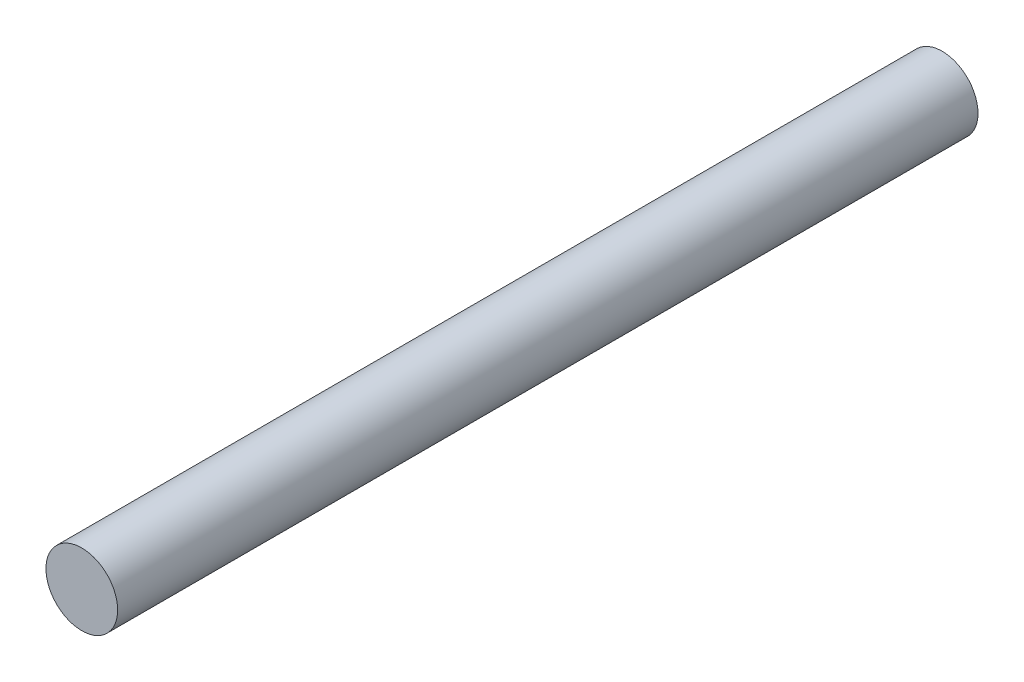
SolidWorks part; units mm, degrees
material "Plain Carbon Steel"
ref_plane "Front Plane" through (0, 0, 0) normal (0, 0, 1) x (1, 0, 0)
ref_plane "Top Plane" through (0, 0, 0) normal (0, 1, 0) x (1, 0, 0)
ref_plane "Right Plane" through (0, 0, 0) normal (1, 0, 0) x (0, 0, -1)
sketch "Pin Profile Ø6" plane through (0, 0, 0) normal (0, 0, 1) x (1, 0, 0)
  circle A0 centre (0, 0) radius 3
  dimension "D1" = 6
extrude "Pin Body Ø6x72" add sketch "Pin Profile Ø6" along normal mid plane 72
